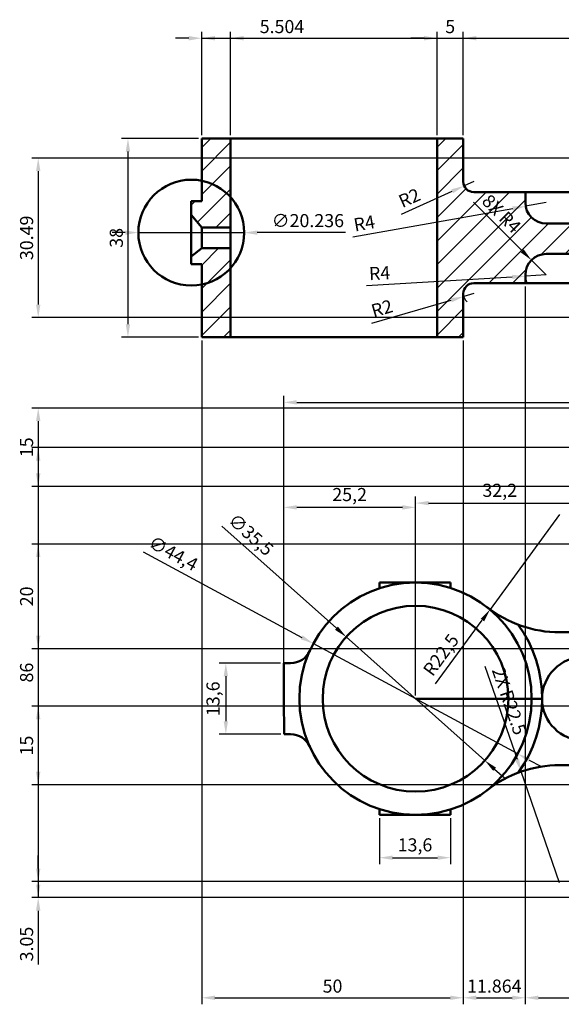
# Model space of a CAD drawing. Units: millimetres. Extents: x 1594 to 1992, y 1694 to 1927.
# Tile 1 of 4: x 1594 to 1698, y 1694 to 1882. Entities that reach past the tile are written whole.
import ezdxf

# ---------------------------------------------------------------- set-up
doc = ezdxf.new("R2010")
doc.units = ezdxf.units.MM
for name, color, linetype, lineweight in [('M-DIMS', 2, 'Continuous', 25), ('M-HATC', 8, 'Continuous', 18), ('M-OUTL', 7, 'Continuous', 50)]:
    doc.layers.add(name, color=color, linetype=linetype, lineweight=lineweight)
doc.styles.get("Standard").update_dxf_attribs({"font": 'arial.ttf'})
doc.dimstyles.new('ISO-25', dxfattribs={"dimtxt": 2.5, "dimasz": 2.5, "dimexe": 1.25, "dimexo": 0.625, "dimtad": 1, "dimtxsty": 'Standard', "dimcen": 2.5, "dimadec": 0, "dimazin": 0, "dimtfac": 1, "dimtmove": 0, "dimatfit": 3, "dimfxl": 1, "dimarcsym": 0})

# ---------------------------------------------------------------- blocks, each defined once
blk = doc.blocks.new('*D1')
at = {"layer": 'Defpoints', "color": 0, "transparency": 16777216}
for p in [(1628.84, 1859.58), (1614.73, 1821.58), (1628.84, 1821.58)]:
    blk.add_point(p, dxfattribs=at)
at = {"layer": 'M-DIMS', "color": 0, "lineweight": -2, "transparency": 16777216}
for p, q in [((1628.21, 1859.58), (1613.48, 1859.58)), ((1614.73, 1857.08), (1614.73, 1824.08)), ((1628.21, 1821.58), (1613.48, 1821.58))]:
    blk.add_line(p, q, dxfattribs=at)
at = {"layer": 'M-DIMS', "color": 0, "transparency": 16777216}
for points in [[(1614.31, 1857.08), (1615.15, 1857.08), (1614.73, 1859.58)], [(1614.31, 1824.08), (1615.15, 1824.08), (1614.73, 1821.58)]]:
    blk.add_solid(points, dxfattribs=at)
at = {"layer": 'M-DIMS', "color": 0, "transparency": 16777216, "insert": (1612.83, 1840.58), "char_height": 2.5, "attachment_point": 5, "rotation": 90}
blk.add_mtext('38', dxfattribs=at)
blk = doc.blocks.new('*D4')
at = {"layer": 'Defpoints', "color": 0, "transparency": 16777216}
for p in [(1679.01, 1850.5), (1680.84, 1851.32)]:
    blk.add_point(p, dxfattribs=at)
at = {"layer": 'M-DIMS', "color": 0, "lineweight": -2, "transparency": 16777216}
for p, q in [((1680.84, 1851.32), (1679.01, 1850.5)), ((1667.04, 1845.13), (1676.73, 1849.48))]:
    blk.add_line(p, q, dxfattribs=at)
at = {"layer": 'M-DIMS', "color": 0, "transparency": 16777216}
blk.add_solid([(1676.56, 1849.86), (1676.9, 1849.1), (1679.01, 1850.5)], dxfattribs=at)
at = {"layer": 'M-DIMS', "color": 0, "transparency": 16777216, "insert": (1668.67, 1847.92), "char_height": 2.5, "attachment_point": 5, "rotation": 24.1694}
blk.add_mtext('R2', dxfattribs=at)
blk = doc.blocks.new('*D9')
at = {"layer": 'Defpoints', "color": 0, "transparency": 16777216}
for p in [(1690.76, 1846.62), (1694.7, 1847.32)]:
    blk.add_point(p, dxfattribs=at)
at = {"layer": 'M-DIMS', "color": 0, "lineweight": -2, "transparency": 16777216}
for p, q in [((1657.7, 1840.75), (1688.3, 1846.18)), ((1694.7, 1847.32), (1690.76, 1846.62))]:
    blk.add_line(p, q, dxfattribs=at)
at = {"layer": 'M-DIMS', "color": 0, "transparency": 16777216}
blk.add_solid([(1688.23, 1846.59), (1688.38, 1845.77), (1690.76, 1846.62)], dxfattribs=at)
at = {"layer": 'M-DIMS', "color": 0, "transparency": 16777216, "insert": (1659.97, 1843.05), "char_height": 2.5, "attachment_point": 5, "rotation": 10.074}
blk.add_mtext('R4', dxfattribs=at)
blk = doc.blocks.new('*D10')
at = {"layer": 'Defpoints', "color": 0, "transparency": 16777216}
for p in [(1690.71, 1833.26), (1694.7, 1833.49)]:
    blk.add_point(p, dxfattribs=at)
at = {"layer": 'M-DIMS', "color": 0, "lineweight": -2, "transparency": 16777216}
for p, q in [((1660.34, 1831.49), (1688.21, 1833.12)), ((1694.7, 1833.49), (1690.71, 1833.26))]:
    blk.add_line(p, q, dxfattribs=at)
blk.add_arc((1694.7, 1833.49), 4, 180, 201.2458, dxfattribs=at)
at = {"layer": 'M-DIMS', "color": 0, "transparency": 16777216}
blk.add_solid([(1688.19, 1833.53), (1688.24, 1832.7), (1690.71, 1833.26)], dxfattribs=at)
at = {"layer": 'M-DIMS', "color": 0, "transparency": 16777216, "insert": (1662.86, 1833.51), "char_height": 2.5, "attachment_point": 5, "rotation": 3.3408}
blk.add_mtext('R4', dxfattribs=at)
blk = doc.blocks.new('*D11')
at = {"layer": 'Defpoints', "color": 0, "transparency": 16777216}
for p in [(1678.92, 1829.36), (1680.84, 1829.92)]:
    blk.add_point(p, dxfattribs=at)
at = {"layer": 'M-DIMS', "color": 0, "lineweight": -2, "transparency": 16777216}
for p, q in [((1680.84, 1829.92), (1678.92, 1829.36)), ((1661.37, 1824.25), (1676.52, 1828.66))]:
    blk.add_line(p, q, dxfattribs=at)
blk.add_arc((1680.84, 1829.92), 2, 180, 232.0518, dxfattribs=at)
at = {"layer": 'M-DIMS', "color": 0, "transparency": 16777216}
blk.add_solid([(1676.4, 1829.06), (1676.64, 1828.26), (1678.92, 1829.36)], dxfattribs=at)
at = {"layer": 'M-DIMS', "color": 0, "transparency": 16777216, "insert": (1663.37, 1826.79), "char_height": 2.5, "attachment_point": 5, "rotation": 16.2419}
blk.add_mtext('R2', dxfattribs=at)
blk = doc.blocks.new('*D13')
at = {"layer": 'Defpoints', "color": 0, "transparency": 16777216}
for p in [(1701.91, 1789.89), (1701.91, 1760.5), (1669.71, 1752.5)]:
    blk.add_point(p, dxfattribs=at)
at = {"layer": 'M-DIMS', "color": 0, "lineweight": -2, "transparency": 16777216}
for p, q in [((1669.71, 1753.13), (1669.71, 1791.14)), ((1672.21, 1789.89), (1699.41, 1789.89)), ((1701.91, 1761.13), (1701.91, 1791.14))]:
    blk.add_line(p, q, dxfattribs=at)
at = {"layer": 'M-DIMS', "color": 0, "transparency": 16777216}
for points in [[(1672.21, 1790.3), (1672.21, 1789.47), (1669.71, 1789.89)], [(1699.41, 1790.3), (1699.41, 1789.47), (1701.91, 1789.89)]]:
    blk.add_solid(points, dxfattribs=at)
at = {"layer": 'M-DIMS', "color": 0, "transparency": 16777216, "insert": (1685.81, 1792.01), "char_height": 2.5, "attachment_point": 5}
blk.add_mtext('32,2', dxfattribs=at)
blk = doc.blocks.new('*D15')
at = {"layer": 'Defpoints', "color": 0, "transparency": 16777216}
for p in [(1644.51, 1789.07), (1644.51, 1752.5), (1669.71, 1752.5)]:
    blk.add_point(p, dxfattribs=at)
at = {"layer": 'M-DIMS', "color": 0, "lineweight": -2, "transparency": 16777216}
for p, q in [((1644.51, 1753.13), (1644.51, 1790.32)), ((1669.71, 1753.13), (1669.71, 1790.32)), ((1667.21, 1789.07), (1647.01, 1789.07))]:
    blk.add_line(p, q, dxfattribs=at)
at = {"layer": 'M-DIMS', "color": 0, "transparency": 16777216}
for points in [[(1647.01, 1789.49), (1647.01, 1788.65), (1644.51, 1789.07)], [(1667.21, 1789.49), (1667.21, 1788.65), (1669.71, 1789.07)]]:
    blk.add_solid(points, dxfattribs=at)
at = {"layer": 'M-DIMS', "color": 0, "transparency": 16777216, "insert": (1657.11, 1791.2), "char_height": 2.5, "attachment_point": 5}
blk.add_mtext('25,2', dxfattribs=at)
blk = doc.blocks.new('*D16')
at = {"layer": 'Defpoints', "color": 0, "transparency": 16777216}
for p in [(1840.91, 1809.14), (1644.51, 1752.5), (1840.91, 1752.5)]:
    blk.add_point(p, dxfattribs=at)
at = {"layer": 'M-DIMS', "color": 0, "lineweight": -2, "transparency": 16777216}
for p, q in [((1644.51, 1753.13), (1644.51, 1810.39)), ((1840.91, 1753.13), (1840.91, 1810.39)), ((1647.01, 1809.14), (1838.41, 1809.14))]:
    blk.add_line(p, q, dxfattribs=at)
at = {"layer": 'M-DIMS', "color": 0, "transparency": 16777216}
for points in [[(1647.01, 1809.56), (1647.01, 1808.72), (1644.51, 1809.14)], [(1838.41, 1809.56), (1838.41, 1808.72), (1840.91, 1809.14)]]:
    blk.add_solid(points, dxfattribs=at)
at = {"layer": 'M-DIMS', "color": 0, "transparency": 16777216, "insert": (1742.71, 1811.27), "char_height": 2.5, "attachment_point": 5}
blk.add_mtext('196,4', dxfattribs=at)
blk = doc.blocks.new('*D22')
at = {"layer": 'Defpoints', "color": 0, "transparency": 16777216}
for p in [(1662.81, 1730.3), (1676.41, 1730.3), (1676.41, 1722.12)]:
    blk.add_point(p, dxfattribs=at)
at = {"layer": 'M-DIMS', "color": 0, "lineweight": -2, "transparency": 16777216}
for p, q in [((1662.81, 1729.68), (1662.81, 1720.87)), ((1676.41, 1729.68), (1676.41, 1720.87)), ((1665.31, 1722.12), (1673.91, 1722.12))]:
    blk.add_line(p, q, dxfattribs=at)
at = {"layer": 'M-DIMS', "color": 0, "transparency": 16777216}
for points in [[(1665.31, 1722.54), (1665.31, 1721.71), (1662.81, 1722.12)], [(1673.91, 1722.54), (1673.91, 1721.71), (1676.41, 1722.12)]]:
    blk.add_solid(points, dxfattribs=at)
at = {"layer": 'M-DIMS', "color": 0, "transparency": 16777216, "insert": (1669.61, 1724.25), "char_height": 2.5, "attachment_point": 5}
blk.add_mtext('13,6', dxfattribs=at)
blk = doc.blocks.new('*D23')
at = {"layer": 'Defpoints', "color": 0, "transparency": 16777216}
for p in [(1644.51, 1759.3), (1633.44, 1745.7), (1644.58, 1745.7)]:
    blk.add_point(p, dxfattribs=at)
at = {"layer": 'M-DIMS', "color": 0, "lineweight": -2, "transparency": 16777216}
for p, q in [((1643.88, 1759.3), (1632.19, 1759.3)), ((1633.44, 1756.8), (1633.44, 1748.2)), ((1643.95, 1745.7), (1632.19, 1745.7))]:
    blk.add_line(p, q, dxfattribs=at)
at = {"layer": 'M-DIMS', "color": 0, "transparency": 16777216}
for points in [[(1633.03, 1756.8), (1633.86, 1756.8), (1633.44, 1759.3)], [(1633.03, 1748.2), (1633.86, 1748.2), (1633.44, 1745.7)]]:
    blk.add_solid(points, dxfattribs=at)
at = {"layer": 'M-DIMS', "color": 0, "transparency": 16777216, "insert": (1631.32, 1752.5), "char_height": 2.5, "attachment_point": 5, "rotation": 90}
blk.add_mtext('13,6', dxfattribs=at)
blk = doc.blocks.new('*D25')
at = {"layer": 'Defpoints', "color": 0, "transparency": 16777216}
for p in [(1697.26, 1787.7), (1683.96, 1769.56)]:
    blk.add_point(p, dxfattribs=at)
at = {"layer": 'M-DIMS', "color": 0, "lineweight": -2, "transparency": 16777216}
for p, q in [((1697.26, 1787.7), (1683.96, 1769.56)), ((1673.54, 1755.34), (1682.48, 1767.54))]:
    blk.add_line(p, q, dxfattribs=at)
at = {"layer": 'M-DIMS', "color": 0, "transparency": 16777216}
blk.add_solid([(1682.15, 1767.79), (1682.82, 1767.29), (1683.96, 1769.56)], dxfattribs=at)
at = {"layer": 'M-DIMS', "color": 0, "transparency": 16777216, "insert": (1674.83, 1760.69), "char_height": 2.5, "attachment_point": 5, "rotation": 53.7676}
blk.add_mtext('R22,5', dxfattribs=at)
blk = doc.blocks.new('*D26')
at = {"layer": 'Defpoints', "color": 0, "transparency": 16777216}
for p in [(1650.16, 1763.04), (1689.25, 1741.97)]:
    blk.add_point(p, dxfattribs=at)
at = {"layer": 'M-DIMS', "color": 0, "lineweight": -2, "transparency": 16777216}
for p, q in [((1617.63, 1780.57), (1647.96, 1764.22)), ((1689.25, 1741.97), (1650.16, 1763.04)), ((1691.45, 1740.79), (1693.65, 1739.6))]:
    blk.add_line(p, q, dxfattribs=at)
at = {"layer": 'M-DIMS', "color": 0, "transparency": 16777216}
for points in [[(1648.16, 1764.59), (1647.77, 1763.86), (1650.16, 1763.04)], [(1691.65, 1741.15), (1691.25, 1740.42), (1689.25, 1741.97)]]:
    blk.add_solid(points, dxfattribs=at)
at = {"layer": 'M-DIMS', "color": 0, "transparency": 16777216, "insert": (1623.26, 1780), "char_height": 2.5, "attachment_point": 5, "rotation": 331.6806}
blk.add_mtext('∅44,4', dxfattribs=at)
blk = doc.blocks.new('*D27')
at = {"layer": 'Defpoints', "color": 0, "transparency": 16777216}
for p in [(1656.46, 1764.31), (1682.96, 1740.7)]:
    blk.add_point(p, dxfattribs=at)
at = {"layer": 'M-DIMS', "color": 0, "lineweight": -2, "transparency": 16777216}
for p, q in [((1632.69, 1785.49), (1654.59, 1765.98)), ((1682.96, 1740.7), (1656.46, 1764.31)), ((1684.82, 1739.03), (1686.69, 1737.37))]:
    blk.add_line(p, q, dxfattribs=at)
at = {"layer": 'M-DIMS', "color": 0, "transparency": 16777216}
for points in [[(1654.87, 1766.29), (1654.31, 1765.67), (1656.46, 1764.31)], [(1685.1, 1739.34), (1684.55, 1738.72), (1682.96, 1740.7)]]:
    blk.add_solid(points, dxfattribs=at)
at = {"layer": 'M-DIMS', "color": 0, "transparency": 16777216, "insert": (1638.04, 1783.63), "char_height": 2.5, "attachment_point": 5, "rotation": 318.294}
blk.add_mtext('∅35,5', dxfattribs=at)
blk = doc.blocks.new('*D40')
at = {"layer": 'Defpoints', "color": 0, "transparency": 16777216}
for p in [(1810.91, 1800.5), (1597.57, 1714.5), (1810.91, 1714.5)]:
    blk.add_point(p, dxfattribs=at)
at = {"layer": 'M-DIMS', "color": 0, "lineweight": -2, "transparency": 16777216}
for p, q in [((1810.28, 1800.5), (1596.32, 1800.5)), ((1597.57, 1798), (1597.57, 1717)), ((1810.28, 1714.5), (1596.32, 1714.5))]:
    blk.add_line(p, q, dxfattribs=at)
at = {"layer": 'M-DIMS', "color": 0, "transparency": 16777216}
for points in [[(1597.15, 1798), (1597.99, 1798), (1597.57, 1800.5)], [(1597.15, 1717), (1597.99, 1717), (1597.57, 1714.5)]]:
    blk.add_solid(points, dxfattribs=at)
at = {"layer": 'M-DIMS', "color": 0, "transparency": 16777216, "insert": (1595.67, 1757.5), "char_height": 2.5, "attachment_point": 5, "rotation": 90}
blk.add_mtext('86', dxfattribs=at)
blk = doc.blocks.new('*D41')
at = {"layer": 'Defpoints', "color": 0, "transparency": 16777216}
for p in [(1810.91, 1717.55), (1597.57, 1714.5), (1810.91, 1714.5)]:
    blk.add_point(p, dxfattribs=at)
at = {"layer": 'M-DIMS', "color": 0, "lineweight": -2, "transparency": 16777216}
for p, q in [((1597.57, 1720.05), (1597.57, 1722.55)), ((1810.28, 1717.55), (1596.32, 1717.55)), ((1597.57, 1717.55), (1597.57, 1714.5)), ((1810.28, 1714.5), (1596.32, 1714.5)), ((1597.57, 1712), (1597.57, 1701.74))]:
    blk.add_line(p, q, dxfattribs=at)
at = {"layer": 'M-DIMS', "color": 0, "transparency": 16777216}
for points in [[(1597.15, 1720.05), (1597.99, 1720.05), (1597.57, 1717.55)], [(1597.15, 1712), (1597.99, 1712), (1597.57, 1714.5)]]:
    blk.add_solid(points, dxfattribs=at)
at = {"layer": 'M-DIMS', "color": 0, "transparency": 16777216, "insert": (1595.67, 1705.62), "char_height": 2.5, "attachment_point": 5, "rotation": 90}
blk.add_mtext('3.05', dxfattribs=at)
blk = doc.blocks.new('*D44')
at = {"layer": 'Defpoints', "color": 0, "transparency": 16777216}
for p in [(1932.03, 1782.06), (1597.57, 1762.06), (1932.03, 1762.06)]:
    blk.add_point(p, dxfattribs=at)
at = {"layer": 'M-DIMS', "color": 0, "lineweight": -2, "transparency": 16777216}
for p, q in [((1931.4, 1782.06), (1596.32, 1782.06)), ((1597.57, 1779.56), (1597.57, 1764.56)), ((1931.4, 1762.06), (1596.32, 1762.06))]:
    blk.add_line(p, q, dxfattribs=at)
at = {"layer": 'M-DIMS', "color": 0, "transparency": 16777216}
for points in [[(1597.15, 1779.56), (1597.99, 1779.56), (1597.57, 1782.06)], [(1597.15, 1764.56), (1597.99, 1764.56), (1597.57, 1762.06)]]:
    blk.add_solid(points, dxfattribs=at)
at = {"layer": 'M-DIMS', "color": 0, "transparency": 16777216, "insert": (1595.67, 1772.06), "char_height": 2.5, "attachment_point": 5, "rotation": 90}
blk.add_mtext('20', dxfattribs=at)
blk = doc.blocks.new('*D45')
at = {"layer": 'Defpoints', "color": 0, "transparency": 16777216}
for p in [(1922.03, 1808.06), (1597.57, 1793.06), (1922.03, 1793.06)]:
    blk.add_point(p, dxfattribs=at)
at = {"layer": 'M-DIMS', "color": 0, "lineweight": -2, "transparency": 16777216}
for p, q in [((1921.4, 1808.06), (1596.32, 1808.06)), ((1597.57, 1805.56), (1597.57, 1795.56)), ((1921.4, 1793.06), (1596.32, 1793.06))]:
    blk.add_line(p, q, dxfattribs=at)
at = {"layer": 'M-DIMS', "color": 0, "transparency": 16777216}
for points in [[(1597.15, 1805.56), (1597.99, 1805.56), (1597.57, 1808.06)], [(1597.15, 1795.56), (1597.99, 1795.56), (1597.57, 1793.06)]]:
    blk.add_solid(points, dxfattribs=at)
at = {"layer": 'M-DIMS', "color": 0, "transparency": 16777216, "insert": (1595.67, 1800.56), "char_height": 2.5, "attachment_point": 5, "rotation": 90}
blk.add_mtext('15', dxfattribs=at)
blk = doc.blocks.new('*D46')
at = {"layer": 'Defpoints', "color": 0, "transparency": 16777216}
for p in [(1922.03, 1751.06), (1597.57, 1736.06), (1922.03, 1736.06)]:
    blk.add_point(p, dxfattribs=at)
at = {"layer": 'M-DIMS', "color": 0, "lineweight": -2, "transparency": 16777216}
for p, q in [((1921.4, 1751.06), (1596.32, 1751.06)), ((1597.57, 1748.56), (1597.57, 1738.56)), ((1921.4, 1736.06), (1596.32, 1736.06))]:
    blk.add_line(p, q, dxfattribs=at)
at = {"layer": 'M-DIMS', "color": 0, "transparency": 16777216}
for points in [[(1597.15, 1748.56), (1597.99, 1748.56), (1597.57, 1751.06)], [(1597.15, 1738.56), (1597.99, 1738.56), (1597.57, 1736.06)]]:
    blk.add_solid(points, dxfattribs=at)
at = {"layer": 'M-DIMS', "color": 0, "transparency": 16777216, "insert": (1595.67, 1743.56), "char_height": 2.5, "attachment_point": 5, "rotation": 90}
blk.add_mtext('15', dxfattribs=at)
blk = doc.blocks.new('*D47')
at = {"layer": 'Defpoints', "color": 0, "transparency": 16777216}
for p in [(1834.84, 1878.73), (1628.84, 1859.58), (1834.84, 1859.58)]:
    blk.add_point(p, dxfattribs=at)
at = {"layer": 'M-DIMS', "color": 0, "lineweight": -2, "transparency": 16777216}
for p, q in [((1628.84, 1860.2), (1628.84, 1879.98)), ((1834.84, 1860.2), (1834.84, 1879.98)), ((1631.34, 1878.73), (1832.34, 1878.73))]:
    blk.add_line(p, q, dxfattribs=at)
at = {"layer": 'M-DIMS', "color": 0, "transparency": 16777216}
for points in [[(1631.34, 1879.15), (1631.34, 1878.31), (1628.84, 1878.73)], [(1832.34, 1879.15), (1832.34, 1878.31), (1834.84, 1878.73)]]:
    blk.add_solid(points, dxfattribs=at)
at = {"layer": 'M-DIMS', "color": 0, "transparency": 16777216, "insert": (1731.84, 1880.63), "char_height": 2.5, "attachment_point": 5}
blk.add_mtext('206', dxfattribs=at)
blk = doc.blocks.new('*D48')
at = {"layer": 'Defpoints', "color": 0, "transparency": 16777216}
for p in [(1628.84, 1821.58), (1678.84, 1821.58), (1678.84, 1695.35)]:
    blk.add_point(p, dxfattribs=at)
at = {"layer": 'M-DIMS', "color": 0, "lineweight": -2, "transparency": 16777216}
for p, q in [((1628.84, 1820.95), (1628.84, 1694.1)), ((1678.84, 1820.95), (1678.84, 1694.1)), ((1631.34, 1695.35), (1676.34, 1695.35))]:
    blk.add_line(p, q, dxfattribs=at)
at = {"layer": 'M-DIMS', "color": 0, "transparency": 16777216}
for points in [[(1631.34, 1695.77), (1631.34, 1694.94), (1628.84, 1695.35)], [(1676.34, 1695.77), (1676.34, 1694.94), (1678.84, 1695.35)]]:
    blk.add_solid(points, dxfattribs=at)
at = {"layer": 'M-DIMS', "color": 0, "transparency": 16777216, "insert": (1653.84, 1697.26), "char_height": 2.5, "attachment_point": 5}
blk.add_mtext('50', dxfattribs=at)
blk = doc.blocks.new('*D49')
at = {"layer": 'Defpoints', "color": 0, "transparency": 16777216}
for p in [(1690.7, 1831.92), (1678.84, 1821.58), (1690.7, 1695.35)]:
    blk.add_point(p, dxfattribs=at)
at = {"layer": 'M-DIMS', "color": 0, "lineweight": -2, "transparency": 16777216}
for p, q in [((1690.7, 1831.3), (1690.7, 1694.1)), ((1678.84, 1820.95), (1678.84, 1694.1)), ((1681.34, 1695.35), (1688.2, 1695.35))]:
    blk.add_line(p, q, dxfattribs=at)
at = {"layer": 'M-DIMS', "color": 0, "transparency": 16777216}
for points in [[(1681.34, 1695.77), (1681.34, 1694.94), (1678.84, 1695.35)], [(1688.2, 1695.77), (1688.2, 1694.94), (1690.7, 1695.35)]]:
    blk.add_solid(points, dxfattribs=at)
at = {"layer": 'M-DIMS', "color": 0, "transparency": 16777216, "insert": (1684.77, 1697.26), "char_height": 2.5, "attachment_point": 5}
blk.add_mtext('11.864', dxfattribs=at)
blk = doc.blocks.new('*D50')
at = {"layer": 'Defpoints', "color": 0, "transparency": 16777216}
for p in [(1690.7, 1831.92), (1789.63, 1831.92), (1789.63, 1695.35)]:
    blk.add_point(p, dxfattribs=at)
at = {"layer": 'M-DIMS', "color": 0, "lineweight": -2, "transparency": 16777216}
for p, q in [((1690.7, 1831.3), (1690.7, 1694.1)), ((1789.63, 1831.3), (1789.63, 1694.1)), ((1693.2, 1695.35), (1787.13, 1695.35))]:
    blk.add_line(p, q, dxfattribs=at)
at = {"layer": 'M-DIMS', "color": 0, "transparency": 16777216}
for points in [[(1693.2, 1695.77), (1693.2, 1694.94), (1690.7, 1695.35)], [(1787.13, 1695.77), (1787.13, 1694.94), (1789.63, 1695.35)]]:
    blk.add_solid(points, dxfattribs=at)
at = {"layer": 'M-DIMS', "color": 0, "transparency": 16777216, "insert": (1740.17, 1697.26), "char_height": 2.5, "attachment_point": 5}
blk.add_mtext('98.93', dxfattribs=at)
blk = doc.blocks.new('*D52')
at = {"layer": 'Defpoints', "color": 0, "transparency": 16777216}
for p in [(1834.84, 1855.83), (1597.57, 1825.34), (1834.84, 1825.34)]:
    blk.add_point(p, dxfattribs=at)
at = {"layer": 'M-DIMS', "color": 0, "lineweight": -2, "transparency": 16777216}
for p, q in [((1834.21, 1855.83), (1596.32, 1855.83)), ((1597.57, 1853.33), (1597.57, 1827.84)), ((1834.21, 1825.34), (1596.32, 1825.34))]:
    blk.add_line(p, q, dxfattribs=at)
at = {"layer": 'M-DIMS', "color": 0, "transparency": 16777216}
for points in [[(1597.15, 1853.33), (1597.99, 1853.33), (1597.57, 1855.83)], [(1597.15, 1827.84), (1597.99, 1827.84), (1597.57, 1825.34)]]:
    blk.add_solid(points, dxfattribs=at)
at = {"layer": 'M-DIMS', "color": 0, "transparency": 16777216, "insert": (1595.67, 1840.58), "char_height": 2.5, "attachment_point": 5, "rotation": 90}
blk.add_mtext('30.49', dxfattribs=at)
blk = doc.blocks.new('*D54')
at = {"layer": 'Defpoints', "color": 0, "transparency": 16777216}
for p in [(1634.34, 1878.73), (1628.84, 1859.58), (1634.34, 1859.58)]:
    blk.add_point(p, dxfattribs=at)
at = {"layer": 'M-DIMS', "color": 0, "lineweight": -2, "transparency": 16777216}
for p, q in [((1628.84, 1860.2), (1628.84, 1879.98)), ((1634.34, 1860.2), (1634.34, 1879.98)), ((1626.34, 1878.73), (1623.84, 1878.73)), ((1628.84, 1878.73), (1634.34, 1878.73)), ((1636.84, 1878.73), (1649.02, 1878.73))]:
    blk.add_line(p, q, dxfattribs=at)
at = {"layer": 'M-DIMS', "color": 0, "transparency": 16777216}
for points in [[(1626.34, 1879.15), (1626.34, 1878.31), (1628.84, 1878.73)], [(1636.84, 1879.15), (1636.84, 1878.31), (1634.34, 1878.73)]]:
    blk.add_solid(points, dxfattribs=at)
at = {"layer": 'M-DIMS', "color": 0, "transparency": 16777216, "insert": (1644.18, 1880.63), "char_height": 2.5, "attachment_point": 5}
blk.add_mtext('5.504', dxfattribs=at)
blk = doc.blocks.new('*D55')
at = {"layer": 'Defpoints', "color": 0, "transparency": 16777216}
for p in [(1678.84, 1878.73), (1673.84, 1859.58), (1678.84, 1859.58)]:
    blk.add_point(p, dxfattribs=at)
at = {"layer": 'M-DIMS', "color": 0, "lineweight": -2, "transparency": 16777216}
for p, q in [((1673.84, 1860.2), (1673.84, 1879.98)), ((1678.84, 1860.2), (1678.84, 1879.98)), ((1671.34, 1878.73), (1668.84, 1878.73)), ((1673.84, 1878.73), (1678.84, 1878.73)), ((1681.34, 1878.73), (1683.84, 1878.73))]:
    blk.add_line(p, q, dxfattribs=at)
at = {"layer": 'M-DIMS', "color": 0, "transparency": 16777216}
for points in [[(1671.34, 1879.15), (1671.34, 1878.31), (1673.84, 1878.73)], [(1681.34, 1879.15), (1681.34, 1878.31), (1678.84, 1878.73)]]:
    blk.add_solid(points, dxfattribs=at)
at = {"layer": 'M-DIMS', "color": 0, "transparency": 16777216, "insert": (1676.34, 1880.63), "char_height": 2.5, "attachment_point": 5}
blk.add_mtext('5', dxfattribs=at)
blk = doc.blocks.new('*D58')
at = {"layer": 'Defpoints', "color": 0, "transparency": 16777216}
for p in [(1689.92, 1738.58), (1697.26, 1717.3)]:
    blk.add_point(p, dxfattribs=at)
at = {"layer": 'M-DIMS', "color": 0, "lineweight": -2, "transparency": 16777216}
for p, q in [((1682.98, 1758.7), (1689.11, 1740.94)), ((1697.26, 1717.3), (1689.92, 1738.58))]:
    blk.add_line(p, q, dxfattribs=at)
at = {"layer": 'M-DIMS', "color": 0, "transparency": 16777216}
blk.add_solid([(1689.5, 1741.08), (1688.71, 1740.8), (1689.92, 1738.58)], dxfattribs=at)
at = {"layer": 'M-DIMS', "color": 0, "transparency": 16777216, "insert": (1687.32, 1751.96), "char_height": 2.5, "attachment_point": 5, "rotation": 289.0251}
blk.add_mtext('2X R22.5', dxfattribs=at)
blk = doc.blocks.new('*D64')
at = {"layer": 'Defpoints', "color": 0, "transparency": 16777216}
for p in [(1691.87, 1836.32), (1694.7, 1833.49)]:
    blk.add_point(p, dxfattribs=at)
at = {"layer": 'M-DIMS', "color": 0, "lineweight": -2, "transparency": 16777216}
for p, q in [((1680.81, 1847.39), (1690.11, 1838.09)), ((1694.7, 1833.49), (1691.87, 1836.32))]:
    blk.add_line(p, q, dxfattribs=at)
at = {"layer": 'M-DIMS', "color": 0, "transparency": 16777216}
blk.add_solid([(1690.4, 1838.38), (1689.81, 1837.8), (1691.87, 1836.32)], dxfattribs=at)
at = {"layer": 'M-DIMS', "color": 0, "transparency": 16777216, "insert": (1685.92, 1844.97), "char_height": 2.5, "attachment_point": 5, "rotation": 314.9999}
blk.add_mtext('8X R4', dxfattribs=at)
blk = doc.blocks.new('*D67')
at = {"layer": 'Defpoints', "color": 0, "transparency": 16777216}
for p in [(1616.72, 1841.58), (1636.96, 1841.58)]:
    blk.add_point(p, dxfattribs=at)
at = {"layer": 'M-DIMS', "color": 0, "lineweight": -2, "transparency": 16777216}
for p, q in [((1614.22, 1841.58), (1611.72, 1841.58)), ((1616.72, 1841.58), (1636.96, 1841.58)), ((1656.3, 1841.58), (1639.46, 1841.58))]:
    blk.add_line(p, q, dxfattribs=at)
at = {"layer": 'M-DIMS', "color": 0, "transparency": 16777216}
for points in [[(1614.22, 1842), (1614.22, 1841.16), (1616.72, 1841.58)], [(1639.46, 1842), (1639.46, 1841.16), (1636.96, 1841.58)]]:
    blk.add_solid(points, dxfattribs=at)
at = {"layer": 'M-DIMS', "color": 0, "transparency": 16777216, "insert": (1649.13, 1843.55), "char_height": 2.5, "attachment_point": 5, "rotation": 0.0016}
blk.add_mtext('∅20.236', dxfattribs=at)

msp = doc.modelspace()

# ---------------------------------------------------------------- hatches: boundary and pattern name
at = {"layer": 'M-HATC'}
h = msp.add_hatch(dxfattribs=at)
h.set_pattern_fill('ANSI31', color=256)
h.paths.add_polyline_path([(1634.343, 1859.5797), (1628.8392, 1859.5797), (1628.8392, 1847.5797), (1626.8392, 1847.5797), (1626.8392, 1844.9915), (1628.8392, 1842.5797), (1634.343, 1842.5797)])
h.paths.add_polyline_path([(1634.343, 1838.5797), (1628.8392, 1838.5797), (1626.8392, 1837.0361), (1626.8392, 1835.5797), (1628.8392, 1835.5797), (1628.8392, 1821.5797), (1634.343, 1821.5797)])
h = msp.add_hatch(dxfattribs=at)
h.set_pattern_fill('ANSI31', color=256)
h.paths.add_polyline_path([(1804.8392, 1855.8272), (1799.8392, 1859.5797), (1799.8392, 1854.5797), (1799.8392, 1851.3192, -0.41421356), (1797.8392, 1849.3192), (1789.6319, 1849.3192), (1789.6319, 1847.3189, -0.41421356), (1785.6319, 1843.3189), (1694.7029, 1843.3189, -0.41421356), (1690.7029, 1847.3189), (1690.7029, 1849.3192), (1680.8392, 1849.3192, -0.41421356), (1678.8392, 1851.3192), (1678.8392, 1859.5797), (1673.8392, 1859.5797), (1673.8392, 1821.5797), (1678.8392, 1821.5797), (1678.8392, 1829.9212, -0.41421356), (1680.8392, 1831.9212), (1690.7029, 1831.9212), (1690.7029, 1833.4941, -0.41421356), (1694.7029, 1837.4941), (1785.6319, 1837.4941, -0.41421356), (1789.6319, 1833.4941), (1789.6319, 1831.9212), (1797.8392, 1831.9212, -0.41421356), (1799.8392, 1829.9212), (1799.8392, 1826.5797), (1799.8392, 1821.5797), (1804.8392, 1825.339)])

# ---------------------------------------------------------------- linework, layer by layer
at = {"layer": 'M-OUTL'}
for p, q in [((1628.8392, 1859.5797), (1628.8392, 1847.5797)), ((1678.8392, 1859.5797), (1628.8392, 1859.5797)), ((1628.8392, 1859.5797), (1628.8392, 1847.5797)), ((1634.343, 1859.5797), (1634.343, 1821.5797)), ((1678.8392, 1859.5797), (1673.8392, 1859.5797)), ((1673.8392, 1859.5797), (1673.8392, 1821.5797)), ((1678.8392, 1851.3192), (1678.8392, 1859.5797)), ((1678.8392, 1859.5797), (1678.8392, 1854.5797)), ((1680.8392, 1849.3192), (1797.8392, 1849.3192)), ((1690.7029, 1847.3189), (1690.7029, 1849.3192)), ((1628.8392, 1847.5797), (1626.8392, 1847.5797)), ((1626.8392, 1847.5797), (1626.8392, 1835.5797)), ((1628.8392, 1842.5797), (1626.8392, 1844.9915)), ((1634.343, 1842.5797), (1628.8392, 1842.5797)), ((1628.8392, 1842.5797), (1628.8392, 1838.5797)), ((1634.343, 1840.5797), (1634.343, 1842.5797)), ((1694.7029, 1843.3189), (1785.6319, 1843.3189)), ((1628.8392, 1838.5797), (1626.8392, 1837.0361)), ((1628.8392, 1838.5797), (1634.343, 1838.5797)), ((1694.7029, 1837.4941), (1785.6319, 1837.4941)), ((1626.8392, 1835.5797), (1628.8392, 1835.5797)), ((1628.8392, 1835.5797), (1628.8392, 1821.5797)), ((1690.7029, 1833.4941), (1690.7029, 1831.9212)), ((1797.8392, 1831.9212), (1680.8392, 1831.9212)), ((1678.8392, 1821.5797), (1678.8392, 1829.9212)), ((1628.8392, 1821.5797), (1678.8392, 1821.5797)), ((1669.7068, 1774.7048), (1662.8068, 1774.7048)), ((1662.8068, 1774.7048), (1662.8068, 1773.6053)), ((1669.7068, 1774.7048), (1676.4068, 1774.7048)), ((1676.4068, 1773.6696), (1676.4068, 1774.7048)), ((1755.3068, 1765.2048), (1697.2577, 1765.2048)), ((1644.5068, 1752.5048), (1644.5068, 1759.3048)), ((1644.5068, 1759.3048), (1645.8363, 1759.3048)), ((1644.5768, 1745.7048), (1644.5068, 1752.5048)), ((1669.7068, 1752.5048), (1693.9068, 1752.5048)), ((1645.8363, 1745.7048), (1644.5768, 1745.7048)), ((1755.3068, 1739.8048), (1697.2577, 1739.8048)), ((1662.8068, 1730.3048), (1662.8068, 1731.4043)), ((1676.4068, 1731.34), (1676.4068, 1730.3048)), ((1669.7068, 1730.3048), (1662.8068, 1730.3048)), ((1669.7068, 1730.3048), (1676.4068, 1730.3048))]:
    msp.add_line(p, q, dxfattribs=at)
for centre, radius in [((1626.8392, 1841.5797), 10.1182), ((1669.7068, 1752.5048), 22.2), ((1669.7068, 1752.5048), 17.75)]:
    msp.add_circle(centre, radius, dxfattribs=at)
for centre, radius, start, end in [((1680.8392, 1851.3192), 2, 180, 270), ((1694.7029, 1847.3189), 4, 180, 270), ((1694.7029, 1833.4941), 4, 90, 180), ((1680.8392, 1829.9212), 2, 90, 180), ((1697.2577, 1787.7048), 22.5, 231.949893, 270), ((1669.7068, 1752.5048), 24.2, 324.259235, 35.740765), ((1645.8363, 1763.3048), 4, 270, 335.656025), ((1701.9068, 1752.5048), 8, 90, 270), ((1645.8363, 1741.7048), 4, 24.343975, 90), ((1697.2577, 1717.3048), 22.5, 90, 128.050107)]:
    msp.add_arc(centre, radius, start, end, dxfattribs=at)

# ---------------------------------------------------------------- dimensions: what is measured, and where the dimension line sits
at = {"layer": 'M-DIMS'}
for base, p1, p2, override, picture, middle in [((1634.343, 1878.7297), (1628.8392, 1859.5797), (1634.343, 1859.5797), {"dimdec": 3, "dimlfac": 1, "dimrnd": 0, "dimzin": 0, "dimdsep": 46, "dimlunit": 2}, '*D54', (1644.181, 1880.6312)), ((1834.8392, 1878.7297), (1628.8392, 1859.5797), (1834.8392, 1859.5797), {"dimdec": 0, "dimlfac": 1, "dimrnd": 0, "dimzin": 0, "dimdsep": 46, "dimlunit": 2}, '*D47', (1731.8392, 1880.6312)), ((1678.8392, 1878.7297), (1673.8392, 1859.5797), (1678.8392, 1859.5797), {"dimdec": 0, "dimlfac": 1, "dimrnd": 0, "dimzin": 0, "dimdsep": 46, "dimlunit": 2}, '*D55', (1676.3392, 1880.626)), ((1690.7029, 1695.3548), (1678.8392, 1821.5797), (1690.7029, 1831.9212), {"dimdec": 3, "dimlfac": 1, "dimrnd": 0, "dimzin": 0, "dimdsep": 46, "dimlunit": 2}, '*D49', (1684.771, 1697.2562)), ((1789.6319, 1695.3548), (1690.7029, 1831.9212), (1789.6319, 1831.9212), {"dimdec": 2, "dimlfac": 1, "dimrnd": 0, "dimzin": 0, "dimdsep": 46, "dimlunit": 2}, '*D50', (1740.1674, 1697.2571)), ((1678.8392, 1695.3548), (1628.8392, 1821.5797), (1678.8392, 1821.5797), {"dimdec": 0, "dimlfac": 1, "dimrnd": 0, "dimzin": 0, "dimdsep": 46, "dimlunit": 2}, '*D48', (1653.8392, 1697.2562)), ((1840.9068, 1809.14), (1644.5068, 1752.5048), (1840.9068, 1752.5048), {"dimclrd": 0, "dimclre": 0, "dimclrt": 0}, '*D16', (1742.7068, 1811.2674)), ((1701.9068, 1789.8851), (1669.7068, 1752.5048), (1701.9068, 1760.5048), {"dimclrd": 0, "dimclre": 0, "dimclrt": 0}, '*D13', (1685.8068, 1792.0125)), ((1644.5068, 1789.0691), (1669.7068, 1752.5048), (1644.5068, 1752.5048), {"dimclrd": 0, "dimclre": 0, "dimclrt": 0}, '*D15', (1657.1068, 1791.1964)), ((1676.4068, 1722.1217), (1662.8068, 1730.3048), (1676.4068, 1730.3048), {"dimclrd": 0, "dimclre": 0, "dimclrt": 0}, '*D22', (1669.6068, 1724.2491))]:
    dim = msp.add_linear_dim(base=base, p1=p1, p2=p2, dimstyle='ISO-25', override=override, dxfattribs=at)
    dim.commit()
    dim.dimension.update_dxf_attribs({"geometry": picture, "text_midpoint": middle})
for base, p1, p2, override, picture, middle in [((1614.73, 1821.5797), (1628.8392, 1859.5797), (1628.8392, 1821.5797), {"dimclrd": 0, "dimclre": 0, "dimclrt": 0}, '*D1', (1612.8277, 1840.5797)), ((1597.571, 1825.339), (1834.8392, 1855.8272), (1834.8392, 1825.339), {"dimdec": 2, "dimlfac": 1, "dimrnd": 0, "dimzin": 0, "dimdsep": 46, "dimlunit": 2}, '*D52', (1595.6687, 1840.5831)), ((1597.571, 1793.0568), (1922.03, 1808.0568), (1922.03, 1793.0568), {"dimdec": 0, "dimlfac": 1, "dimrnd": 0, "dimzin": 0, "dimdsep": 46, "dimlunit": 2}, '*D45', (1595.6695, 1800.5568)), ((1597.571, 1714.5048), (1810.9068, 1800.5048), (1810.9068, 1714.5048), {"dimdec": 0, "dimlfac": 1, "dimrnd": 0, "dimzin": 0, "dimdsep": 46, "dimlunit": 2}, '*D40', (1595.6695, 1757.5048)), ((1597.571, 1762.0568), (1932.03, 1782.0568), (1932.03, 1762.0568), {"dimdec": 0, "dimlfac": 1, "dimrnd": 0, "dimzin": 0, "dimdsep": 46, "dimlunit": 2}, '*D44', (1595.6695, 1772.0568)), ((1633.4439, 1745.7048), (1644.5068, 1759.3048), (1644.5768, 1745.7048), {"dimclrd": 0, "dimclre": 0, "dimclrt": 0}, '*D23', (1631.3165, 1752.5048)), ((1597.571, 1736.0568), (1922.03, 1751.0568), (1922.03, 1736.0568), {"dimdec": 0, "dimlfac": 1, "dimrnd": 0, "dimzin": 0, "dimdsep": 46, "dimlunit": 2}, '*D46', (1595.6695, 1743.5568)), ((1597.571, 1714.5048), (1810.9068, 1717.5546), (1810.9068, 1714.5048), {"dimdec": 2, "dimlfac": 1, "dimrnd": 0, "dimzin": 0, "dimdsep": 46, "dimlunit": 2}, '*D41', (1595.6687, 1705.6243))]:
    dim = msp.add_linear_dim(base=base, p1=p1, p2=p2, angle=90, dimstyle='ISO-25', override=override, dxfattribs=at)
    dim.commit()
    dim.dimension.update_dxf_attribs({"geometry": picture, "text_midpoint": middle})
for center, mpoint, picture, middle in [((1680.8392, 1851.3192), (1679.0145, 1850.5003), '*D4', (1669.4354, 1846.2015)), ((1694.7029, 1847.3189), (1690.7645, 1846.6192), '*D9', (1660.2999, 1841.2069)), ((1694.7029, 1833.4941), (1690.7097, 1833.261), '*D10', (1662.9716, 1831.6418)), ((1680.8392, 1829.9212), (1678.919, 1829.3618), '*D11', (1663.8958, 1824.9853)), ((1697.2577, 1787.7048), (1683.9588, 1769.5557), '*D25', (1676.543, 1759.4353))]:
    dim = msp.add_radius_dim(center=center, mpoint=mpoint, dimstyle='ISO-25', override={"dimclrd": 0, "dimclre": 0, "dimclrt": 0}, dxfattribs=at)
    dim.commit()
    dim.dimension.update_dxf_attribs({"geometry": picture, "text_midpoint": middle, "dimtype": 164})
dim = msp.add_radius_dim(center=(1694.7029, 1833.4941), mpoint=(1691.8744, 1836.3226), text='8X <>', dimstyle='ISO-25', override={"dimdec": 0, "dimlfac": 1, "dimrnd": 0, "dimzin": 0, "dimdsep": 46, "dimlunit": 2}, dxfattribs=at)
dim.commit()
dim.dimension.update_dxf_attribs({"geometry": '*D64', "text_midpoint": (1685.9194, 1844.9667)})
dim = msp.add_diameter_dim_2p(p1=(1616.721, 1841.5794), p2=(1636.9573, 1841.58), dimstyle='ISO-25', override={"dimdec": 3, "dimlfac": 1, "dimrnd": 0, "dimzin": 0, "dimdsep": 46, "dimlunit": 2}, dxfattribs=at)
dim.commit()
dim.dimension.update_dxf_attribs({"geometry": '*D67', "text_midpoint": (1649.1308, 1841.5803)})
for p1, p2, picture, middle in [((1682.9584, 1740.6956), (1656.4552, 1764.314), '*D27', (1636.6011, 1782.0072)), ((1689.2499, 1741.9734), (1650.1638, 1763.0362), '*D26', (1622.2274, 1778.0906))]:
    dim = msp.add_diameter_dim_2p(p1=p1, p2=p2, dimstyle='ISO-25', override={"dimclrd": 0, "dimclre": 0, "dimclrt": 0}, dxfattribs=at)
    dim.commit()
    dim.dimension.update_dxf_attribs({"geometry": picture, "text_midpoint": middle, "dimtype": 163})
dim = msp.add_radius_dim(center=(1697.2577, 1717.3048), mpoint=(1689.9231, 1738.5757), text='2X <>', dimstyle='ISO-25', override={"dimdec": 1, "dimlfac": 1, "dimrnd": 0, "dimzin": 0, "dimdsep": 46, "dimlunit": 2}, dxfattribs=at)
dim.commit()
dim.dimension.update_dxf_attribs({"geometry": '*D58', "text_midpoint": (1685.5223, 1751.3383), "dimtype": 164})

doc.saveas('drawing.dxf')
